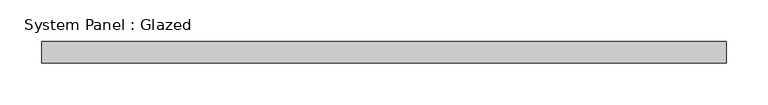
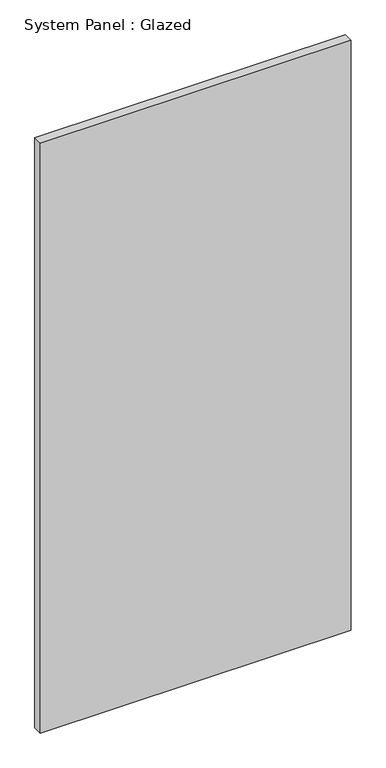
"""IFC4 building model written with IfcOpenShell, lengths in millimetres: plate geometry, System Panel : Glazed."""

from ifc_helpers import new_model, si_unit, origin, origin_with_axes, place, context, project, spatial, polyline, outline, extrude, source, transform, mapped, element, save


def system_panel_glazed_6e362244(model_context):
    return source(origin(), model_context, "Body", "SweptSolid", [
        extrude(outline(polyline([(409.575, 19.05), (-409.575, 19.05), (-409.575, 44.45), (409.575, 44.45), (409.575, 19.05)])), origin_with_axes(), (0.0, 0.0, 1.0), 1643.7328538),
    ])


if __name__ == "__main__":
    model = new_model("IFC4")
    model_context = context("Model", 3, world=origin())
    ifc_project = project(units=[si_unit("LENGTHUNIT", "METRE", prefix="MILLI")], contexts=[model_context])
    site = spatial("IfcSite", under=ifc_project)
    building = spatial("IfcBuilding", under=site)
    placement = place(None, origin())
    system_panel_glazed_shape = system_panel_glazed_6e362244(model_context)
    element("IfcPlate", 1, ObjectType="System Panel : Glazed", at=placement, inside=building, context=model_context, shape_type="MappedRepresentation", body=[
        mapped(system_panel_glazed_shape, transform((0.0, 0.0, 0.0), x_axis=(1.0, 0.0, 0.0), y_axis=(0.0, 1.0, 0.0), z_axis=(0.0, 0.0, 1.0))),
    ])
    save(model, "model.ifc")

# Revit data of these elements
# Type "System Panel : Glazed"
#   Construction Type Id = "GSP4R"
#   Analytic Construction = "1/8 in Pilkington single glazing"
#   Visual Light Transmittance = 0.9
#   Solar Heat Gain Coefficient = 0.86
#   Heat Transfer Coefficient (U) = 1.18115 BTU/(h·ft²·°F)
#   Define Thermal Properties by = 1
# Element 1 (IfcPlate, "System Panel : Glazed")
#   Materials on its faces: "Glass"
# Materials
#   "Glass": class "Glass", colour RGB 0 128 192, transparency 0.75, Description = "Soda Lime Glass", Cost = 0
